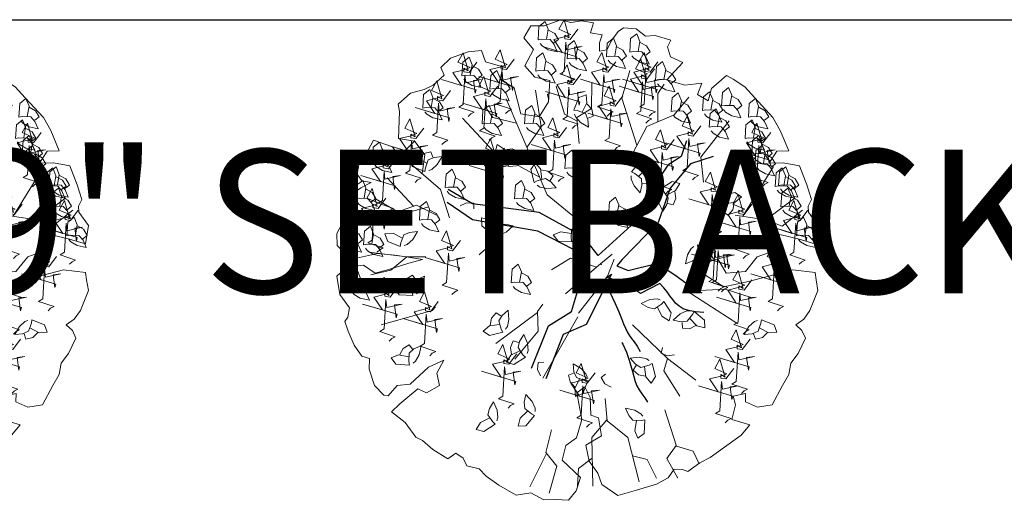
# Model space of a CAD drawing. Units: inches. Extents: x 2831 to 4250, y 1103 to 1797.
# Tile 8 of 15: x 3614 to 3676, y 1690 to 1721. Entities that reach past the tile are written whole.
import ezdxf

# ---------------------------------------------------------------- set-up
doc = ezdxf.new("R2010")
doc.units = ezdxf.units.IN
for name, color, linetype, lineweight in [('A-ANNO-DIMS', 2, 'Continuous', 18), ('A-ANNO-TEXT', 7, 'Continuous', 18), ('A-WALL-PATT', 252, 'Continuous', 13), ('ARBOL', 30, 'Continuous', 13), ('C-PROP', 7, 'Continuous', 25)]:
    doc.layers.add(name, color=color, linetype=linetype, lineweight=lineweight)
doc.layers.add('TALLO', color=36, linetype='Continuous')
doc.styles.get("Standard").update_dxf_attribs({"font": 'arial.ttf'})
doc.dimstyles.new('ISO-25', dxfattribs={"dimtxt": 9, "dimasz": 2.5, "dimexe": 1.25, "dimexo": 0.625, "dimtad": 1, "dimdec": 1, "dimlunit": 3, "dimtxsty": 'Standard', "dimcen": 2.5, "dimadec": 0, "dimazin": 0, "dimtfac": 1, "dimtdec": 1, "dimtmove": 0, "dimatfit": 3, "dimfxl": 1, "dimarcsym": 0})

# ---------------------------------------------------------------- blocks, each defined once
blk = doc.blocks.new('fresno')
at = {"layer": 'ARBOL'}
for p, q in [((2.96, 0.991), (3.575, 1.984)), ((-3.638, 1.194), (-4.164, 1.76)), ((-1.151, -0.932), (-1.99, -1.556)), ((-0.974, -3.757), (-1.31, -4.423))]:
    blk.add_line(p, q, dxfattribs=at)
blk.add_lwpolyline([(0.823, 4.745), (0.566, 4.764), (0.459, 4.687), (0.336, 4.518), (0.233, 4.322), (0.087, 4.298), (0.091, 4.464), (0.14, 4.621), (-0.09, 4.659), (-0.033, 4.863), (-0.264, 4.901), (-0.483, 4.866), (-0.686, 4.924), (-1.021, 4.801), (-1.288, 4.8), (-1.431, 4.563), (-1.234, 4.327), (-1.406, 4), (-1.205, 3.778), (-0.909, 3.705), (-0.931, 3.283), (-1.122, 2.983), (-1.491, 3.043), (-1.619, 3.562), (-1.9, 3.727), (-1.851, 3.982), (-2.197, 4.084), (-2.278, 4.31), (-2.543, 4.283), (-2.896, 4.152), (-3.091, 3.971), (-3.022, 3.817), (-3.244, 3.617), (-3.424, 3.528), (-3.697, 3.455), (-3.946, 3.236), (-3.922, 3.09), (-3.94, 2.548), (-3.617, 2.495), (-3.927, 2.19), (-4.062, 2.379), (-4.443, 2.512), (-4.546, 2.316), (-4.73, 2.062), (-4.767, 1.832), (-4.671, 1.698), (-4.486, 1.667), (-4.693, 1.559), (-4.854, 1.444), (-4.934, 1.102), (-5.037, 0.905), (-5.175, 0.644), (-5.166, 0.406), (-5.024, 0.264), (-4.781, 0.153), (-4.363, 0.249), (-4.014, 0.215), (-3.783, 0.177), (-3.46, 0.124), (-3.733, 0.051), (-4.132, -0.073), (-4.404, -0.146), (-4.639, 0.011), (-4.977, -0.028), (-5.172, -0.209), (-5.113, -0.574), (-4.921, -0.843), (-4.951, -1.027), (-5.012, -1.112), (-4.95, -1.311), (-4.83, -1.592), (-4.676, -1.807), (-4.518, -1.856), (-4.529, -2.068), (-4.417, -2.394), (-4.236, -2.59), (-4.143, -2.605), (-3.967, -2.397), (-3.703, -2.37), (-3.339, -2.027), (-3.032, -1.889), (-3.169, -2.15), (-3.115, -2.396), (-3.376, -2.542), (-3.552, -2.466), (-3.909, -2.762), (-4.077, -2.924), (-3.804, -3.135), (-3.592, -3.43), (-3.461, -3.499), (-3.253, -3.676), (-2.953, -3.867), (-2.792, -3.752), (-2.642, -3.848), (-2.572, -4.001), (-2.323, -4.066), (-2.18, -4.208), (-1.926, -4.392), (-1.58, -4.591), (-1.288, -4.545), (-1.027, -4.683), (-0.788, -4.675), (-0.531, -4.693), (-0.382, -4.505), (-0.29, -4.236), (-0.66, -3.891), (-0.588, -3.595), (-0.374, -3.441), (-0.267, -3.079), (-0.368, -2.541), (-0.208, -2.426), (-0.099, -2.633), (-0.087, -2.991), (0.071, -3.04), (0.129, -3.405), (-0.185, -3.59), (-0.119, -3.909), (0.055, -4.151), (0.136, -4.377), (0.456, -4.596), (0.828, -4.491), (1.227, -4.368), (1.461, -4.241), (1.583, -4.071), (1.748, -4.075), (1.86, -4.117), (2.101, -3.944), (2.308, -3.836), (2.925, -3.393), (3.101, -3.185), (2.74, -3.078), (2.812, -2.782), (2.769, -2.61), (3.015, -2.555), (3.012, -2.721), (3.254, -2.832), (3.546, -2.785), (3.752, -2.393), (3.882, -2.177), (3.92, -1.947), (4.069, -1.758), (4.214, -1.451), (4.144, -1.297), (4.021, -1.182), (4.182, -1.067), (4.304, -0.897), (4.464, -0.497), (4.429, -0.279), (4.406, -0.133), (3.964, -0.083), (3.074, -0.315), (2.582, -0.424), (2.217, -0.197), (2.136, 0.029), (2.462, 0.141), (2.628, -0.147), (3.012, -0.116), (3.249, 0.177), (3.602, 0.308), (3.701, 0.623), (4.089, 0.535), (4.404, 0.436), (4.464, 0.805), (4.272, 1.074), (4.267, 1.193), (4.336, 1.324), (4.243, 1.623), (4.092, 2.003), (3.769, 2.057), (3.485, 2.056), (3.642, 2.291), (3.88, 2.299), (3.71, 2.706), (3.563, 2.967), (3.201, 3.358), (3.001, 3.581), (2.766, 3.738), (2.635, 3.807), (2.332, 3.549), (2.268, 3.299), (2.052, 3.429), (2.136, 3.652), (1.798, 3.613), (1.437, 3.72), (1.755, 4.071), (1.513, 4.182), (1.451, 4.381), (1.519, 4.512), (1.204, 4.611), (1.012, 4.596)], close=True, dxfattribs=at)
for points in [[(-1.104, 4.45), (-1.063, 4.399), (-0.939, 4.325), (-0.757, 4.285), (-0.82, 4.431), (-0.903, 4.527), (-1.075, 4.533), (-1.143, 4.521), (-1.126, 4.792), (-1.002, 4.891), (-0.939, 4.738), (-0.975, 4.535)], [(-0.346, 4.735), (-0.501, 4.528), (-0.605, 4.545), (-0.605, 4.614), (-0.519, 4.563), (-0.622, 4.925), (-0.726, 4.735), (-0.484, 4.632), (-0.622, 4.58), (-0.829, 4.528), (-0.657, 4.27), (-1.053, 4.39), (-0.363, 4.183), (-0.381, 4.114), (-0.415, 4.373), (-0.26, 4.39), (-0.57, 4.321), (-0.588, 4.476), (-0.622, 3.89), (-0.708, 3.839), (-0.398, 3.735), (-0.467, 3.701), (-0.519, 3.649)], [(-0.935, 4.717), (-0.809, 4.65), (-0.736, 4.529), (-0.824, 4.459)], [(0.263, 4.114), (0.304, 4.063), (0.429, 3.989), (0.611, 3.948), (0.547, 4.095), (0.465, 4.191), (0.293, 4.197), (0.225, 4.185), (0.242, 4.456), (0.366, 4.555), (0.428, 4.402), (0.393, 4.199)], [(0.734, 4.203), (0.775, 4.152), (0.9, 4.078), (1.082, 4.038), (1.018, 4.185), (0.936, 4.281), (0.763, 4.287), (0.696, 4.274), (0.712, 4.546), (0.837, 4.645), (0.899, 4.491), (0.863, 4.289)], [(-0.521, 4.069), (-0.48, 4.018), (-0.356, 3.944), (-0.174, 3.904), (-0.237, 4.051), (-0.32, 4.146), (-0.492, 4.152), (-0.56, 4.14), (-0.543, 4.411), (-0.419, 4.511), (-0.356, 4.357), (-0.392, 4.154)], [(0.433, 4.381), (0.558, 4.314), (0.631, 4.193), (0.544, 4.122)], [(0.904, 4.471), (1.029, 4.404), (1.102, 4.282), (1.015, 4.212)], [(-2.368, 4.073), (-2.523, 3.866), (-2.627, 3.883), (-2.627, 3.952), (-2.541, 3.9), (-2.644, 4.262), (-2.748, 4.073), (-2.506, 3.969), (-2.644, 3.918), (-2.851, 3.866), (-2.679, 3.607), (-3.075, 3.728), (-2.385, 3.521), (-2.403, 3.452), (-2.437, 3.711), (-2.282, 3.728), (-2.592, 3.659), (-2.61, 3.814), (-2.644, 3.228), (-2.73, 3.176), (-2.42, 3.073), (-2.489, 3.038), (-2.541, 2.987)], [(-2.629, 3.733), (-2.588, 3.682), (-2.463, 3.608), (-2.281, 3.568), (-2.345, 3.715), (-2.427, 3.81), (-2.6, 3.816), (-2.667, 3.804), (-2.651, 4.075), (-2.526, 4.175), (-2.464, 4.021), (-2.5, 3.818)], [(-1.623, 4.132), (-1.778, 3.925), (-1.882, 3.942), (-1.882, 4.011), (-1.795, 3.959), (-1.899, 4.321), (-2.002, 4.132), (-1.761, 4.028), (-1.899, 3.977), (-2.106, 3.925), (-1.933, 3.666), (-2.33, 3.787), (-1.64, 3.58), (-1.657, 3.511), (-1.692, 3.77), (-1.537, 3.787), (-1.847, 3.718), (-1.864, 3.873), (-1.899, 3.287), (-1.985, 3.235), (-1.675, 3.132), (-1.744, 3.097), (-1.795, 3.046)], [(-1.149, 3.822), (-1.108, 3.771), (-0.983, 3.697), (-0.802, 3.657), (-0.865, 3.804), (-0.948, 3.9), (-1.12, 3.906), (-1.188, 3.893), (-1.171, 4.165), (-1.047, 4.264), (-0.984, 4.111), (-1.02, 3.908)], [(-0.352, 4.337), (-0.226, 4.269), (-0.153, 4.148), (-0.241, 4.078)], [(0.413, 4.08), (0.258, 3.873), (0.154, 3.89), (0.154, 3.959), (0.241, 3.908), (0.137, 4.27), (0.034, 4.08), (0.275, 3.977), (0.137, 3.925), (-0.07, 3.873), (0.103, 3.614), (-0.294, 3.735), (0.396, 3.528), (0.379, 3.459), (0.344, 3.718), (0.499, 3.735), (0.189, 3.666), (0.172, 3.821), (0.137, 3.235), (0.051, 3.183), (0.361, 3.08), (0.292, 3.046), (0.241, 2.994)], [(1.259, 4.08), (1.103, 3.873), (1, 3.89), (1, 3.959), (1.086, 3.908), (0.982, 4.27), (0.879, 4.08), (1.12, 3.977), (0.982, 3.925), (0.775, 3.873), (0.948, 3.614), (0.551, 3.735), (1.241, 3.528), (1.224, 3.459), (1.189, 3.718), (1.345, 3.735), (1.034, 3.666), (1.017, 3.821), (0.982, 3.235), (0.896, 3.183), (1.207, 3.08), (1.138, 3.046), (1.086, 2.994)], [(-2.459, 4), (-2.334, 3.933), (-2.261, 3.812), (-2.348, 3.742)], [(-0.287, 3.833), (-0.442, 3.626), (-0.546, 3.643), (-0.546, 3.712), (-0.46, 3.661), (-0.563, 4.023), (-0.667, 3.833), (-0.425, 3.73), (-0.563, 3.678), (-0.77, 3.626), (-0.598, 3.367), (-0.995, 3.488), (-0.304, 3.281), (-0.322, 3.212), (-0.356, 3.471), (-0.201, 3.488), (-0.511, 3.419), (-0.529, 3.574), (-0.563, 2.988), (-0.649, 2.936), (-0.339, 2.833), (-0.408, 2.799), (-0.46, 2.747)], [(-0.98, 4.09), (-0.854, 4.023), (-0.781, 3.901), (-0.869, 3.831)], [(1.189, 3.942), (1.034, 3.735), (0.931, 3.752), (0.931, 3.821), (1.017, 3.77), (0.913, 4.132), (0.81, 3.942), (1.051, 3.839), (0.913, 3.787), (0.706, 3.735), (0.879, 3.477), (0.482, 3.597), (1.172, 3.39), (1.155, 3.321), (1.12, 3.58), (1.276, 3.597), (0.965, 3.528), (0.948, 3.683), (0.913, 3.097), (0.827, 3.046), (1.138, 2.942), (1.069, 2.908), (1.017, 2.856)], [(1.25, 3.643), (1.291, 3.592), (1.416, 3.518), (1.597, 3.478), (1.534, 3.625), (1.451, 3.721), (1.279, 3.727), (1.211, 3.714), (1.228, 3.985), (1.352, 4.085), (1.415, 3.931), (1.379, 3.729)], [(-1.951, 3.597), (-2.106, 3.39), (-2.209, 3.408), (-2.209, 3.477), (-2.123, 3.425), (-2.227, 3.787), (-2.33, 3.597), (-2.089, 3.494), (-2.227, 3.442), (-2.434, 3.39), (-2.261, 3.132), (-2.658, 3.252), (-1.968, 3.046), (-1.985, 2.977), (-2.02, 3.235), (-1.864, 3.252), (-2.175, 3.183), (-2.192, 3.339), (-2.227, 2.752), (-2.313, 2.701), (-2.002, 2.597), (-2.071, 2.563), (-2.123, 2.511)], [(-2.068, 3.464), (-2.027, 3.413), (-1.903, 3.339), (-1.721, 3.299), (-1.784, 3.446), (-1.867, 3.542), (-2.039, 3.547), (-2.107, 3.535), (-2.09, 3.806), (-1.966, 3.906), (-1.903, 3.752), (-1.939, 3.55)], [(0.837, 2.414), (0.533, 3.352), (0.697, 3.906)], [(1.419, 3.911), (1.545, 3.844), (1.618, 3.722), (1.53, 3.652)], [(-2.898, 3.511), (-3.053, 3.304), (-3.157, 3.321), (-3.157, 3.39), (-3.071, 3.339), (-3.174, 3.701), (-3.278, 3.511), (-3.036, 3.408), (-3.174, 3.356), (-3.381, 3.304), (-3.209, 3.046), (-3.605, 3.166), (-2.915, 2.959), (-2.932, 2.89), (-2.967, 3.149), (-2.812, 3.166), (-3.122, 3.097), (-3.14, 3.253), (-3.174, 2.666), (-3.26, 2.615), (-2.95, 2.511), (-3.019, 2.477), (-3.071, 2.425)], [(-1.899, 3.732), (-1.773, 3.664), (-1.7, 3.543), (-1.788, 3.473)], [(-0.358, 2.895), (-0.615, 3.037), (-0.783, 3.596)], [(-0.063, 3.671), (-0.069, 3.151), (-0.364, 2.965), (-0.319, 2.449)], [(0.558, 3.402), (0.403, 3.195), (0.299, 3.212), (0.299, 3.281), (0.386, 3.23), (0.282, 3.592), (0.179, 3.402), (0.42, 3.299), (0.282, 3.247), (0.075, 3.195), (0.248, 2.936), (-0.149, 3.057), (0.541, 2.85), (0.524, 2.781), (0.489, 3.04), (0.644, 3.057), (0.334, 2.988), (0.317, 3.143), (0.282, 2.557), (0.196, 2.505), (0.506, 2.402), (0.437, 2.368), (0.386, 2.316)], [(1.259, 2.882), (1.254, 3.446), (1.381, 3.636)], [(2.573, 3.128), (2.613, 3.077), (2.738, 3.003), (2.92, 2.963), (2.857, 3.11), (2.774, 3.205), (2.602, 3.211), (2.534, 3.199), (2.551, 3.47), (2.675, 3.57), (2.738, 3.416), (2.702, 3.214)], [(-3.413, 3.083), (-3.373, 3.032), (-3.248, 2.958), (-3.066, 2.918), (-3.129, 3.065), (-3.212, 3.161), (-3.384, 3.167), (-3.452, 3.154), (-3.435, 3.425), (-3.311, 3.525), (-3.248, 3.371), (-3.284, 3.169)], [(-1.367, 2.367), (-1.081, 2.78), (-1.193, 3.514)], [(-0.923, 3.449), (-0.951, 3.425), (-0.93, 3.313)], [(-0.41, 3.035), (-0.387, 2.974), (-0.291, 2.865), (-0.131, 2.771), (-0.146, 2.93), (-0.195, 3.047), (-0.357, 3.106), (-0.425, 3.115), (-0.325, 3.368), (-0.176, 3.424), (-0.164, 3.258), (-0.261, 3.077)], [(0.746, 2.242), (1.034, 2.786), (1.584, 3.019), (1.879, 3.374)], [(1.564, 3.016), (1.605, 2.965), (1.729, 2.891), (1.911, 2.851), (1.848, 2.998), (1.765, 3.094), (1.593, 3.099), (1.525, 3.087), (1.542, 3.358), (1.666, 3.458), (1.729, 3.304), (1.693, 3.102)], [(2.191, 3.038), (2.232, 2.987), (2.357, 2.913), (2.539, 2.873), (2.475, 3.02), (2.393, 3.116), (2.221, 3.122), (2.153, 3.109), (2.17, 3.381), (2.294, 3.48), (2.356, 3.326), (2.321, 3.124)], [(2.742, 3.396), (2.868, 3.328), (2.941, 3.207), (2.853, 3.137)], [(-3.244, 3.351), (-3.118, 3.284), (-3.045, 3.162), (-3.133, 3.092)], [(-2.225, 2.77), (-2.184, 2.718), (-2.06, 2.645), (-1.878, 2.604), (-1.941, 2.751), (-2.024, 2.847), (-2.196, 2.853), (-2.264, 2.84), (-2.247, 3.112), (-2.123, 3.211), (-2.06, 3.058), (-2.096, 2.855)], [(-1.575, 2.854), (-2.052, 2.969), (-2.2, 3.178)], [(-0.448, 1), (-0.961, 1.419), (-1.784, 3.341)], [(-1.373, 2.77), (-1.332, 2.718), (-1.208, 2.645), (-1.026, 2.604), (-1.089, 2.751), (-1.172, 2.847), (-1.344, 2.853), (-1.412, 2.84), (-1.395, 3.112), (-1.271, 3.211), (-1.208, 3.058), (-1.244, 2.855)], [(-0.166, 3.238), (-0.068, 3.135), (-0.036, 2.997), (-0.141, 2.957)], [(1.733, 3.284), (1.859, 3.216), (1.932, 3.095), (1.844, 3.025)], [(2.361, 3.306), (2.486, 3.239), (2.559, 3.117), (2.472, 3.047)], [(3.111, 2.904), (3.152, 2.853), (3.276, 2.779), (3.458, 2.739), (3.395, 2.886), (3.312, 2.981), (3.14, 2.987), (3.072, 2.975), (3.089, 3.246), (3.213, 3.346), (3.276, 3.192), (3.24, 2.99)], [(3.28, 3.172), (3.406, 3.104), (3.479, 2.983), (3.391, 2.913)], [(-2.056, 3.037), (-1.93, 2.97), (-1.857, 2.849), (-1.945, 2.778)], [(-0.57, 2.77), (-0.726, 2.563), (-0.829, 2.58), (-0.829, 2.649), (-0.743, 2.597), (-0.846, 2.959), (-0.95, 2.77), (-0.708, 2.666), (-0.846, 2.615), (-1.053, 2.563), (-0.881, 2.304), (-1.278, 2.425), (-0.588, 2.218), (-0.605, 2.149), (-0.639, 2.408), (-0.484, 2.425), (-0.795, 2.356), (-0.812, 2.511), (-0.846, 1.925), (-0.933, 1.873), (-0.622, 1.77), (-0.691, 1.735), (-0.743, 1.684)], [(-1.204, 3.037), (-1.078, 2.97), (-1.005, 2.849), (-1.093, 2.778)], [(2.121, 2.804), (1.966, 2.597), (1.862, 2.615), (1.862, 2.683), (1.949, 2.632), (1.845, 2.994), (1.742, 2.804), (1.983, 2.701), (1.845, 2.649), (1.638, 2.597), (1.811, 2.339), (1.414, 2.459), (2.104, 2.252), (2.087, 2.184), (2.052, 2.442), (2.207, 2.459), (1.897, 2.39), (1.88, 2.546), (1.845, 1.959), (1.759, 1.908), (2.069, 1.804), (2, 1.77), (1.949, 1.718)], [(2.326, 2.702), (2.367, 2.651), (2.492, 2.577), (2.673, 2.537), (2.61, 2.684), (2.527, 2.78), (2.355, 2.786), (2.287, 2.773), (2.304, 3.045), (2.428, 3.144), (2.491, 2.99), (2.455, 2.788)], [(2.495, 2.97), (2.621, 2.903), (2.694, 2.781), (2.606, 2.711)], [(-3.434, 2.752), (-3.59, 2.546), (-3.693, 2.563), (-3.693, 2.632), (-3.607, 2.58), (-3.71, 2.942), (-3.814, 2.752), (-3.572, 2.649), (-3.71, 2.597), (-3.917, 2.546), (-3.745, 2.287), (-4.142, 2.408), (-3.452, 2.201), (-3.469, 2.132), (-3.503, 2.39), (-3.348, 2.408), (-3.659, 2.339), (-3.676, 2.494), (-3.71, 1.908), (-3.797, 1.856), (-3.486, 1.753), (-3.555, 1.718), (-3.607, 1.666)], [(-1.112, 1.773), (-2.014, 2.265), (-2.654, 2.957)], [(2.171, 1.674), (2.121, 2.172), (2.689, 2.898)], [(3.519, 2.666), (3.363, 2.459), (3.26, 2.477), (3.26, 2.546), (3.346, 2.494), (3.243, 2.856), (3.139, 2.666), (3.381, 2.563), (3.243, 2.511), (3.036, 2.459), (3.208, 2.201), (2.811, 2.321), (3.501, 2.115), (3.484, 2.046), (3.45, 2.304), (3.605, 2.321), (3.294, 2.252), (3.277, 2.408), (3.243, 1.821), (3.156, 1.77), (3.467, 1.666), (3.398, 1.632), (3.346, 1.58)], [(3.043, 2.478), (3.084, 2.427), (3.209, 2.353), (3.391, 2.313), (3.327, 2.46), (3.245, 2.556), (3.073, 2.562), (3.005, 2.549), (3.022, 2.82), (3.146, 2.92), (3.208, 2.766), (3.173, 2.564)], [(1.586, 2.528), (1.431, 2.321), (1.327, 2.339), (1.327, 2.408), (1.414, 2.356), (1.31, 2.718), (1.207, 2.528), (1.448, 2.425), (1.31, 2.373), (1.103, 2.321), (1.276, 2.063), (0.879, 2.184), (1.569, 1.977), (1.552, 1.908), (1.517, 2.166), (1.673, 2.184), (1.362, 2.115), (1.345, 2.27), (1.31, 1.684), (1.224, 1.632), (1.535, 1.528), (1.466, 1.494), (1.414, 1.442)], [(3.178, 2.165), (3.219, 2.113), (3.344, 2.04), (3.525, 1.999), (3.462, 2.146), (3.379, 2.242), (3.207, 2.248), (3.139, 2.236), (3.156, 2.507), (3.28, 2.606), (3.343, 2.453), (3.307, 2.25)], [(3.213, 2.746), (3.338, 2.679), (3.411, 2.557), (3.324, 2.487)], [(-4.422, 2.03), (-4.381, 1.979), (-4.257, 1.905), (-4.075, 1.865), (-4.138, 2.012), (-4.221, 2.108), (-4.393, 2.114), (-4.461, 2.101), (-4.444, 2.372), (-4.32, 2.472), (-4.257, 2.318), (-4.293, 2.116)], [(-3.468, 1.85), (-3.409, 2.222), (-3.628, 2.505)], [(-1.817, 2.351), (-1.972, 2.144), (-2.075, 2.162), (-2.075, 2.231), (-1.989, 2.179), (-2.093, 2.541), (-2.196, 2.351), (-1.955, 2.248), (-2.093, 2.196), (-2.3, 2.144), (-2.127, 1.886), (-2.524, 2.006), (-1.834, 1.8), (-1.851, 1.731), (-1.886, 1.989), (-1.73, 2.006), (-2.041, 1.937), (-2.058, 2.093), (-2.093, 1.506), (-2.179, 1.455), (-1.868, 1.351), (-1.937, 1.317), (-1.989, 1.265)], [(-1.786, 2.007), (-1.722, 1.99), (-1.578, 2.003), (-1.407, 2.078), (-1.545, 2.159), (-1.668, 2.188), (-1.811, 2.092), (-1.859, 2.042), (-2.004, 2.271), (-1.962, 2.425), (-1.821, 2.337), (-1.731, 2.152)], [(3.245, 1.963), (3.286, 1.912), (3.411, 1.838), (3.593, 1.798), (3.529, 1.945), (3.447, 2.041), (3.274, 2.046), (3.206, 2.034), (3.223, 2.305), (3.347, 2.405), (3.41, 2.251), (3.374, 2.049)], [(3.347, 2.432), (3.473, 2.365), (3.546, 2.244), (3.458, 2.173)], [(-3.986, 2.149), (-4.142, 1.942), (-4.245, 1.959), (-4.245, 2.028), (-4.159, 1.977), (-4.262, 2.339), (-4.366, 2.149), (-4.124, 2.046), (-4.262, 1.994), (-4.47, 1.942), (-4.297, 1.684), (-4.694, 1.804), (-4.004, 1.597), (-4.021, 1.528), (-4.055, 1.787), (-3.9, 1.804), (-4.211, 1.735), (-4.228, 1.89), (-4.262, 1.304), (-4.349, 1.253), (-4.038, 1.149), (-4.107, 1.115), (-4.159, 1.063)], [(-4.253, 2.298), (-4.127, 2.231), (-4.054, 2.109), (-4.142, 2.039)], [(-2.916, 0.958), (-3.096, 1.528), (-3.871, 2.197)], [(-3.331, 1.905), (-3.269, 1.928), (-3.161, 2.024), (-3.066, 2.184), (-3.226, 2.169), (-3.342, 2.121), (-3.401, 1.958), (-3.41, 1.89), (-3.663, 1.99), (-3.719, 2.139), (-3.554, 2.151), (-3.372, 2.054)], [(-3.533, 2.149), (-3.43, 2.247), (-3.292, 2.279), (-3.252, 2.174)], [(-1.806, 2.323), (-1.665, 2.343), (-1.534, 2.287), (-1.564, 2.179)], [(-0.566, 1.873), (-0.525, 1.822), (-0.4, 1.748), (-0.219, 1.708), (-0.282, 1.855), (-0.365, 1.951), (-0.537, 1.957), (-0.605, 1.944), (-0.588, 2.216), (-0.464, 2.315), (-0.401, 2.162), (-0.437, 1.959)], [(3.415, 2.231), (3.54, 2.163), (3.613, 2.042), (3.525, 1.972)], [(-1.164, 1.612), (-1.109, 1.576), (-0.967, 1.544), (-0.782, 1.562), (-0.888, 1.682), (-0.996, 1.748), (-1.162, 1.7), (-1.222, 1.667), (-1.29, 1.93), (-1.203, 2.063), (-1.096, 1.937), (-1.067, 1.733)], [(-0.397, 2.141), (-0.271, 2.074), (-0.198, 1.952), (-0.286, 1.882)], [(0.72, 1.798), (0.723, 1.733), (0.781, 1.6), (0.904, 1.46), (0.939, 1.616), (0.929, 1.742), (0.793, 1.848), (0.73, 1.878), (0.904, 2.088), (1.062, 2.095), (1.023, 1.934), (0.875, 1.791)], [(3.716, 1.537), (3.757, 1.486), (3.882, 1.412), (4.063, 1.372), (4, 1.519), (3.917, 1.615), (3.745, 1.621), (3.677, 1.608), (3.694, 1.88), (3.818, 1.979), (3.881, 1.825), (3.845, 1.623)], [(-2.965, 1.493), (-2.924, 1.441), (-2.799, 1.368), (-2.618, 1.327), (-2.681, 1.474), (-2.764, 1.57), (-2.936, 1.576), (-3.004, 1.564), (-2.987, 1.835), (-2.863, 1.934), (-2.8, 1.781), (-2.836, 1.578)], [(-1.085, 1.919), (-0.945, 1.893), (-0.838, 1.801), (-0.9, 1.707)], [(1.014, 1.915), (1.077, 1.787), (1.064, 1.646), (0.952, 1.64)], [(2.587, 1.684), (2.432, 1.477), (2.328, 1.494), (2.328, 1.563), (2.414, 1.511), (2.311, 1.873), (2.207, 1.684), (2.449, 1.58), (2.311, 1.528), (2.104, 1.477), (2.276, 1.218), (1.88, 1.339), (2.57, 1.132), (2.552, 1.063), (2.518, 1.321), (2.673, 1.339), (2.363, 1.27), (2.345, 1.425), (2.311, 0.839), (2.225, 0.787), (2.535, 0.684), (2.466, 0.649), (2.414, 0.597)], [(3.649, 1.515), (3.69, 1.464), (3.814, 1.39), (3.996, 1.35), (3.933, 1.497), (3.85, 1.592), (3.678, 1.598), (3.61, 1.586), (3.627, 1.857), (3.751, 1.957), (3.814, 1.803), (3.778, 1.601)], [(3.818, 1.783), (3.944, 1.715), (4.017, 1.594), (3.929, 1.524)], [(3.885, 1.805), (4.011, 1.738), (4.084, 1.616), (3.996, 1.546)], [(-4.759, 1.269), (-4.718, 1.217), (-4.593, 1.144), (-4.411, 1.103), (-4.475, 1.25), (-4.557, 1.346), (-4.729, 1.352), (-4.797, 1.339), (-4.78, 1.611), (-4.656, 1.71), (-4.594, 1.557), (-4.629, 1.354)], [(-2.796, 1.76), (-2.67, 1.693), (-2.597, 1.572), (-2.685, 1.501)], [(-1.575, 1.269), (-1.534, 1.217), (-1.409, 1.144), (-1.228, 1.103), (-1.291, 1.25), (-1.373, 1.346), (-1.546, 1.352), (-1.614, 1.339), (-1.597, 1.611), (-1.473, 1.71), (-1.41, 1.557), (-1.446, 1.354)], [(1.283, 1.469), (1.266, 1.405), (1.279, 1.261), (1.354, 1.09), (1.435, 1.228), (1.464, 1.351), (1.368, 1.494), (1.318, 1.542), (1.547, 1.687), (1.7, 1.645), (1.613, 1.504), (1.428, 1.414)], [(-4.193, 1.356), (-4.349, 1.149), (-4.452, 1.166), (-4.452, 1.235), (-4.366, 1.184), (-4.469, 1.546), (-4.573, 1.356), (-4.331, 1.253), (-4.469, 1.201), (-4.677, 1.149), (-4.504, 0.89), (-4.901, 1.011), (-4.211, 0.804), (-4.228, 0.735), (-4.262, 0.994), (-4.107, 1.011), (-4.418, 0.942), (-4.435, 1.097), (-4.469, 0.511), (-4.556, 0.459), (-4.245, 0.356), (-4.314, 0.322), (-4.366, 0.27)], [(-4.589, 1.536), (-4.464, 1.469), (-4.391, 1.348), (-4.478, 1.277)], [(-1.406, 1.536), (-1.28, 1.469), (-1.207, 1.348), (-1.295, 1.277)], [(1.599, 1.489), (1.618, 1.348), (1.563, 1.217), (1.455, 1.247)], [(2.479, 1.34), (2.443, 1.285), (2.411, 1.143), (2.429, 0.958), (2.549, 1.064), (2.615, 1.172), (2.567, 1.338), (2.534, 1.398), (2.797, 1.466), (2.93, 1.379), (2.804, 1.272), (2.6, 1.243)], [(3.139, 1.235), (2.984, 1.028), (2.88, 1.046), (2.88, 1.115), (2.967, 1.063), (2.863, 1.425), (2.759, 1.235), (3.001, 1.132), (2.863, 1.08), (2.656, 1.028), (2.828, 0.77), (2.432, 0.891), (3.122, 0.684), (3.105, 0.615), (3.07, 0.873), (3.225, 0.891), (2.915, 0.822), (2.897, 0.977), (2.863, 0.391), (2.777, 0.339), (3.087, 0.235), (3.018, 0.201), (2.967, 0.149)], [(3.761, 1.112), (3.802, 1.061), (3.926, 0.987), (4.108, 0.947), (4.045, 1.093), (3.962, 1.189), (3.79, 1.195), (3.722, 1.183), (3.739, 1.454), (3.863, 1.553), (3.926, 1.4), (3.89, 1.197)], [(-3.192, 1.017), (-3.578, 1.215), (-3.949, 1.081), (-4.398, 1.339)], [(-3.481, 0.843), (-3.44, 0.792), (-3.315, 0.718), (-3.133, 0.678), (-3.197, 0.825), (-3.279, 0.92), (-3.451, 0.926), (-3.519, 0.914), (-3.502, 1.185), (-3.378, 1.285), (-3.316, 1.131), (-3.351, 0.928)], [(-2.703, 1.201), (-2.575, 1.263), (-2.433, 1.251), (-2.428, 1.139)], [(0.308, 0.933), (0.349, 0.881), (0.474, 0.807), (0.656, 0.767), (0.592, 0.914), (0.51, 1.01), (0.337, 1.016), (0.27, 1.003), (0.286, 1.275), (0.411, 1.374), (0.473, 1.221), (0.437, 1.018)], [(0.478, 1.2), (0.603, 1.133), (0.676, 1.011), (0.589, 0.941)], [(2.786, 1.261), (2.76, 1.121), (2.668, 1.014), (2.574, 1.076)], [(4.01, 1.36), (3.422, 0.918)], [(4.26, 1.115), (4.105, 0.908), (4.002, 0.925), (4.002, 0.994), (4.088, 0.942), (3.984, 1.304), (3.881, 1.115), (4.122, 1.011), (3.984, 0.959), (3.777, 0.908), (3.95, 0.649), (3.553, 0.77), (4.243, 0.563), (4.226, 0.494), (4.191, 0.753), (4.347, 0.77), (4.036, 0.701), (4.019, 0.856), (3.984, 0.27), (3.898, 0.218), (4.209, 0.115), (4.14, 0.08), (4.088, 0.029)], [(3.93, 1.379), (4.056, 1.312), (4.129, 1.191), (4.041, 1.121)], [(-3.354, 1.176), (-4.529, 0.864)], [(-3.311, 1.111), (-3.186, 1.043), (-3.113, 0.922), (-3.2, 0.852)], [(2.808, 1.015), (3.422, 0.918), (3.422, 0.918), (3.748, 0.794), (4.154, 1.111)], [(-5.028, 0.44), (-4.987, 0.388), (-4.862, 0.315), (-4.68, 0.274), (-4.744, 0.421), (-4.826, 0.517), (-4.998, 0.523), (-5.066, 0.511), (-5.049, 0.782), (-4.925, 0.881), (-4.863, 0.728), (-4.898, 0.525)], [(-4.602, 0.35), (-4.561, 0.299), (-4.436, 0.225), (-4.254, 0.185), (-4.318, 0.332), (-4.4, 0.428), (-4.572, 0.433), (-4.64, 0.421), (-4.623, 0.692), (-4.499, 0.792), (-4.437, 0.638), (-4.472, 0.436)], [(-1.981, 0.615), (-1.915, 0.618), (-1.782, 0.676), (-1.643, 0.799), (-1.799, 0.834), (-1.925, 0.824), (-2.031, 0.688), (-2.061, 0.626), (-2.27, 0.799), (-2.278, 0.958), (-2.117, 0.918), (-1.974, 0.77)], [(-0.397, 0.517), (-0.346, 0.557), (-0.272, 0.682), (-0.232, 0.864), (-0.379, 0.801), (-0.474, 0.718), (-0.48, 0.546), (-0.468, 0.478), (-0.739, 0.495), (-0.838, 0.619), (-0.685, 0.682), (-0.482, 0.646)], [(4.075, 0.529), (4.116, 0.478), (4.24, 0.404), (4.422, 0.364), (4.359, 0.511), (4.276, 0.607), (4.104, 0.613), (4.036, 0.6), (4.053, 0.871), (4.177, 0.971), (4.24, 0.817), (4.204, 0.615)], [(4.244, 0.797), (4.37, 0.73), (4.443, 0.608), (4.355, 0.538)], [(-4.858, 0.707), (-4.733, 0.64), (-4.66, 0.519), (-4.747, 0.448)], [(-4.432, 0.618), (-4.307, 0.55), (-4.234, 0.429), (-4.321, 0.359)], [(-3.824, 0.404), (-3.763, 0.427), (-3.654, 0.523), (-3.559, 0.683), (-3.719, 0.668), (-3.835, 0.62), (-3.894, 0.457), (-3.903, 0.389), (-4.156, 0.489), (-4.212, 0.638), (-4.047, 0.65), (-3.865, 0.553)], [(-2.698, 0.509), (-2.854, 0.302), (-2.957, 0.319), (-2.957, 0.388), (-2.871, 0.336), (-2.974, 0.698), (-3.078, 0.509), (-2.836, 0.405), (-2.974, 0.353), (-3.182, 0.302), (-3.009, 0.043), (-3.406, 0.164), (-2.716, -0.043), (-2.733, -0.112), (-2.767, 0.147), (-2.612, 0.164), (-2.923, 0.095), (-2.94, 0.25), (-2.974, -0.336), (-3.061, -0.388), (-2.75, -0.491), (-2.819, -0.526), (-2.871, -0.577)], [(2.639, 0.58), (2.483, 0.373), (2.38, 0.391), (2.38, 0.46), (2.466, 0.408), (2.363, 0.77), (2.259, 0.58), (2.501, 0.477), (2.363, 0.425), (2.156, 0.373), (2.328, 0.115), (1.931, 0.235), (2.621, 0.029), (2.604, -0.04), (2.57, 0.218), (2.725, 0.235), (2.414, 0.166), (2.397, 0.322), (2.363, -0.265), (2.276, -0.316), (2.587, -0.42), (2.518, -0.454), (2.466, -0.506)], [(2.708, 0.563), (2.552, 0.356), (2.449, 0.373), (2.449, 0.442), (2.535, 0.391), (2.432, 0.753), (2.328, 0.563), (2.57, 0.46), (2.432, 0.408), (2.225, 0.356), (2.397, 0.097), (2, 0.218), (2.69, 0.011), (2.673, -0.058), (2.639, 0.201), (2.794, 0.218), (2.483, 0.149), (2.466, 0.304), (2.432, -0.282), (2.345, -0.334), (2.656, -0.437), (2.587, -0.471), (2.535, -0.523)], [(1.978, 0.384), (1.927, 0.343), (1.853, 0.218), (1.813, 0.036), (1.96, 0.1), (2.056, 0.182), (2.061, 0.355), (2.049, 0.422), (2.32, 0.406), (2.42, 0.281), (2.266, 0.219), (2.064, 0.254)], [(-3.394, 0.18), (-3.77, 0.182), (-4.532, 0.27)], [(-2.322, 0.222), (-2.219, 0.321), (-2.081, 0.353), (-2.042, 0.248)], [(-0.596, -0.564), (0.03, -0.026), (0.339, 0.235)], [(2.246, 0.214), (2.178, 0.089), (2.057, 0.016), (1.987, 0.103)], [(3.829, 0.184), (3.674, -0.023), (3.57, -0.006), (3.57, 0.063), (3.657, 0.011), (3.553, 0.373), (3.45, 0.184), (3.691, 0.08), (3.553, 0.029), (3.346, -0.023), (3.519, -0.282), (3.122, -0.161), (3.812, -0.368), (3.795, -0.437), (3.76, -0.178), (3.915, -0.161), (3.605, -0.23), (3.588, -0.075), (3.553, -0.661), (3.467, -0.713), (3.777, -0.816), (3.708, -0.851), (3.657, -0.902)], [(-3.77, 0.182), (-4.09, -0.088), (-4.494, -0.18)], [(-1.642, -0.412), (-1.601, -0.463), (-1.477, -0.537), (-1.295, -0.577), (-1.358, -0.43), (-1.441, -0.334), (-1.613, -0.328), (-1.681, -0.341), (-1.664, -0.069), (-1.54, 0.03), (-1.477, -0.124), (-1.513, -0.326)], [(0.03, -0.026), (-0.491, 0.154), (-0.871, -0.08)], [(0.38, 0.131), (0.248, -0.21), (-0.33, -0.951)], [(-4.871, -0.524), (-4.83, -0.575), (-4.705, -0.649), (-4.523, -0.689), (-4.587, -0.542), (-4.669, -0.446), (-4.841, -0.44), (-4.909, -0.453), (-4.893, -0.181), (-4.768, -0.082), (-4.706, -0.236), (-4.741, -0.438)], [(-3.848, -0.389), (-3.781, -0.264), (-3.659, -0.191), (-3.589, -0.278)], [(-1.473, -0.144), (-1.347, -0.211), (-1.274, -0.333), (-1.362, -0.403)], [(3.139, -0.282), (2.984, -0.489), (2.88, -0.471), (2.88, -0.402), (2.967, -0.454), (2.863, -0.092), (2.759, -0.282), (3.001, -0.385), (2.863, -0.437), (2.656, -0.489), (2.828, -0.747), (2.432, -0.627), (3.122, -0.834), (3.105, -0.902), (3.07, -0.644), (3.225, -0.627), (2.915, -0.696), (2.897, -0.54), (2.863, -1.127), (2.777, -1.178), (3.087, -1.282), (3.018, -1.316), (2.967, -1.368)], [(-4.701, -0.256), (-4.576, -0.323), (-4.503, -0.445), (-4.59, -0.515)], [(-3.952, -0.42), (-4.107, -0.627), (-4.211, -0.609), (-4.211, -0.54), (-4.124, -0.592), (-4.228, -0.23), (-4.331, -0.42), (-4.09, -0.523), (-4.228, -0.575), (-4.435, -0.627), (-4.262, -0.885), (-4.659, -0.765), (-3.969, -0.971), (-3.986, -1.04), (-4.021, -0.782), (-3.866, -0.765), (-4.176, -0.834), (-4.193, -0.678), (-4.228, -1.265), (-4.314, -1.316), (-4.004, -1.42), (-4.073, -1.454), (-4.124, -1.506)], [(-3.58, -0.559), (-3.529, -0.518), (-3.455, -0.393), (-3.415, -0.211), (-3.562, -0.275), (-3.658, -0.357), (-3.664, -0.53), (-3.651, -0.597), (-3.923, -0.581), (-4.022, -0.456), (-3.868, -0.394), (-3.666, -0.43)], [(-3.141, -0.713), (-3.296, -0.92), (-3.4, -0.902), (-3.4, -0.834), (-3.314, -0.885), (-3.417, -0.523), (-3.521, -0.713), (-3.279, -0.816), (-3.417, -0.868), (-3.624, -0.92), (-3.452, -1.178), (-3.848, -1.058), (-3.158, -1.265), (-3.175, -1.333), (-3.21, -1.075), (-3.055, -1.058), (-3.365, -1.127), (-3.383, -0.971), (-3.417, -1.558), (-3.503, -1.609), (-3.193, -1.713), (-3.262, -1.747), (-3.314, -1.799)], [(1.822, -0.495), (2.859, -1.165)], [(1.846, -0.51), (2.605, -0.469), (3.129, -0.637)], [(-1.047, -0.767), (-1.151, -0.913), (-1.144, -1.307), (-1.61, -1.871)], [(1.304, -0.681), (1.241, -0.664), (1.097, -0.678), (0.926, -0.752), (1.064, -0.833), (1.187, -0.862), (1.33, -0.766), (1.377, -0.716), (1.523, -0.945), (1.481, -1.099), (1.34, -1.011), (1.25, -0.826)], [(-3.195, -0.824), (-3.267, -0.898), (-4.285, -1.185)], [(-1.794, -1.268), (-1.758, -1.214), (-1.726, -1.072), (-1.744, -0.887), (-1.865, -0.993), (-1.93, -1.101), (-1.883, -1.266), (-1.85, -1.327), (-2.113, -1.395), (-2.246, -1.307), (-2.119, -1.2), (-1.916, -1.172)], [(-2.101, -1.19), (-2.076, -1.05), (-1.983, -0.943), (-1.889, -1.004)], [(1.903, -0.903), (1.837, -0.905), (1.704, -0.963), (1.565, -1.086), (1.721, -1.122), (1.847, -1.111), (1.953, -0.975), (1.983, -0.913), (2.192, -1.086), (2.2, -1.245), (2.039, -1.205), (1.896, -1.057)], [(-0.346, -1.024), (-1.05, -2.251)], [(2.02, -1.197), (1.891, -1.259), (1.75, -1.247), (1.745, -1.134)], [(3.253, -1.094), (3.192, -1.117), (3.083, -1.213), (2.988, -1.374), (3.148, -1.359), (3.264, -1.31), (3.323, -1.148), (3.332, -1.079), (3.585, -1.179), (3.641, -1.328), (3.476, -1.34), (3.294, -1.244)], [(-1.361, -1.756), (-1.343, -1.693), (-1.357, -1.548), (-1.431, -1.377), (-1.513, -1.515), (-1.542, -1.638), (-1.445, -1.781), (-1.395, -1.829), (-1.625, -1.974), (-1.778, -1.932), (-1.691, -1.791), (-1.506, -1.701)], [(0.748, -1.185), (1.452, -1.855), (2.021, -2.292)], [(3.105, -1.471), (2.949, -1.678), (2.846, -1.661), (2.846, -1.592), (2.932, -1.644), (2.829, -1.282), (2.725, -1.471), (2.967, -1.575), (2.829, -1.627), (2.621, -1.678), (2.794, -1.937), (2.397, -1.816), (3.087, -2.023), (3.07, -2.092), (3.036, -1.833), (3.191, -1.816), (2.88, -1.885), (2.863, -1.73), (2.829, -2.316), (2.742, -2.368), (3.053, -2.471), (2.984, -2.506), (2.932, -2.558)], [(3.455, -1.338), (3.352, -1.437), (3.214, -1.469), (3.175, -1.364)], [(-1.571, -1.764), (-1.726, -1.971), (-1.83, -1.954), (-1.83, -1.885), (-1.744, -1.937), (-1.847, -1.575), (-1.951, -1.764), (-1.709, -1.868), (-1.847, -1.92), (-2.054, -1.971), (-1.882, -2.23), (-2.278, -2.109), (-1.588, -2.316), (-1.605, -2.385), (-1.64, -2.127), (-1.485, -2.109), (-1.795, -2.178), (-1.813, -2.023), (-1.847, -2.609), (-1.933, -2.661), (-1.623, -2.764), (-1.692, -2.799), (-1.744, -2.851)], [(-1.677, -1.776), (-1.696, -1.635), (-1.641, -1.504), (-1.533, -1.534)], [(-3.648, -1.948), (-3.596, -1.907), (-3.523, -1.782), (-3.482, -1.6), (-3.629, -1.664), (-3.725, -1.746), (-3.731, -1.919), (-3.719, -1.986), (-3.99, -1.97), (-4.089, -1.845), (-3.936, -1.783), (-3.733, -1.819)], [(-3.915, -1.778), (-3.848, -1.653), (-3.727, -1.58), (-3.656, -1.667)], [(1.593, -1.781), (1.452, -1.801), (1.322, -1.746), (1.352, -1.637)], [(-1.092, -2.202), (-1.154, -2.074), (-1.142, -1.933), (-1.03, -1.928)], [(-0.001, -2.144), (-0.156, -2.351), (-0.26, -2.333), (-0.26, -2.264), (-0.174, -2.316), (-0.277, -1.954), (-0.381, -2.144), (-0.139, -2.247), (-0.277, -2.299), (-0.484, -2.351), (-0.312, -2.609), (-0.708, -2.489), (-0.018, -2.695), (-0.035, -2.764), (-0.07, -2.506), (0.085, -2.489), (-0.225, -2.558), (-0.243, -2.402), (-0.277, -2.989), (-0.363, -3.04), (-0.053, -3.144), (-0.122, -3.178), (-0.174, -3.23)], [(-0.161, -2.225), (-0.184, -2.163), (-0.28, -2.055), (-0.44, -1.96), (-0.425, -2.12), (-0.376, -2.236), (-0.214, -2.295), (-0.146, -2.304), (-0.246, -2.557), (-0.395, -2.613), (-0.407, -2.448), (-0.31, -2.266)], [(1.086, -1.899), (1.031, -1.863), (0.89, -1.831), (0.704, -1.849), (0.81, -1.969), (0.918, -2.035), (1.084, -1.987), (1.145, -1.954), (1.212, -2.218), (1.125, -2.35), (1.018, -2.224), (0.989, -2.02)], [(1.452, -1.855), (1.379, -2.105), (1.698, -2.609)], [(2.777, -2.058), (2.621, -2.264), (2.518, -2.247), (2.518, -2.178), (2.604, -2.23), (2.501, -1.868), (2.397, -2.058), (2.639, -2.161), (2.501, -2.213), (2.294, -2.264), (2.466, -2.523), (2.069, -2.402), (2.759, -2.609), (2.742, -2.678), (2.708, -2.42), (2.863, -2.402), (2.552, -2.471), (2.535, -2.316), (2.501, -2.902), (2.414, -2.954), (2.725, -3.057), (2.656, -3.092), (2.604, -3.144)], [(-0.405, -2.427), (-0.503, -2.324), (-0.535, -2.186), (-0.43, -2.146)], [(0.319, -2.428), (0.193, -2.361), (0.12, -2.239), (0.208, -2.169)], [(1.007, -2.206), (0.867, -2.181), (0.76, -2.088), (0.822, -1.994)], [(-1.966, -3.1), (-1.949, -3.037), (-1.962, -2.892), (-2.037, -2.722), (-2.118, -2.859), (-2.147, -2.982), (-2.051, -3.125), (-2.001, -3.173), (-2.23, -3.319), (-2.383, -3.277), (-2.296, -3.136), (-2.111, -3.046)], [(-1.201, -2.914), (-1.204, -2.849), (-1.262, -2.716), (-1.385, -2.576), (-1.42, -2.732), (-1.41, -2.858), (-1.274, -2.964), (-1.212, -2.994), (-1.385, -3.204), (-1.544, -3.211), (-1.504, -3.05), (-1.356, -2.907)], [(0.201, -2.655), (0.24, -3.105), (0.657, -3.436), (0.886, -4.322)], [(0.959, -3.012), (0.918, -2.961), (0.793, -2.887), (0.612, -2.847), (0.675, -2.994), (0.758, -3.089), (0.93, -3.095), (0.998, -3.083), (0.981, -3.354), (0.857, -3.453), (0.794, -3.3), (0.83, -3.097)], [(1.399, -2.886), (1.63, -3.612), (1.964, -3.708), (2.084, -3.964)], [(0.238, -3.084), (-0.067, -3.438), (-0.048, -4.412)], [(-0.923, -4.549), (-0.768, -4.012), (-0.99, -3.737), (-0.872, -3.28)], [(1.625, -3.596), (1.438, -3.858), (1.657, -4.248)], [(-0.059, -3.851), (-0.336, -4.054), (-0.355, -4.41)], [(0.752, -3.801), (1.042, -3.878), (1.233, -4.25)]]:
    blk.add_lwpolyline(points, dxfattribs=at)
for p in [(-0.308, 0.101), (0.124, 0.027)]:
    blk.add_point(p, dxfattribs=at)
at = {"layer": 'TALLO'}
for points in [[(1.829, 2.5), (1.722, 2.184), (1.454, 2.012), (1.213, 1.639), (0.944, 1.008), (0.06, 0.204), (-0.234, 0.577), (-1.119, 1.065), (-2.458, 1.237), (-2.941, 1.524)], [(2.364, 2.184), (1.909, 2.041), (1.507, 1.552), (1.266, 0.864), (0.542, 0.125), (0.433, 0.001), (0.662, -0.096), (1.228, 0.045), (1.455, -0.09), (1.644, -0.216), (1.8, -0.33), (1.931, -0.425), (2.042, -0.496), (2.141, -0.539)], [(-1.272, -2.047), (-0.931, -1.203), (-0.475, -0.916), (-0.234, -0.112), (-0.422, 0.318), (-1.146, 0.691), (-2.458, 0.921), (-2.967, 1.266)], [(2.177, -0.932), (2.008, -0.924), (1.873, -0.898), (1.766, -0.859), (1.682, -0.807), (1.613, -0.745), (1.554, -0.676), (1.499, -0.6), (1.442, -0.521), (1.376, -0.44), (1.298, -0.357), (0.908, -0.555), (0.791, -0.474), (0.647, -0.394), (0.474, -0.317), (0.265, -0.244), (0.226, -0.233), (0.328, -0.17), (-0.181, -1.175), (-0.637, -1.375), (-0.985, -2.265)], [(0.219, -0.386), (0.3, -0.544), (0.399, -0.753), (0.473, -0.922), (0.529, -1.057), (0.571, -1.164), (0.607, -1.251), (0.641, -1.324), (0.68, -1.389), (0.729, -1.454), (0.784, -1.525), (0.844, -1.61), (0.903, -1.717)], [(0.538, -1.536), (0.555, -1.568), (0.626, -1.728), (0.678, -1.871), (0.716, -2), (0.747, -2.115), (0.773, -2.219), (0.802, -2.314), (0.837, -2.401), (0.883, -2.483), (0.936, -2.562), (0.994, -2.642), (1.052, -2.727)]]:
    blk.add_lwpolyline(points, dxfattribs=at)
blk = doc.blocks.new('*D77')
at = {"layer": 'A-ANNO-DIMS', "color": 0, "lineweight": -2, "transparency": 16777216}
for p, q in [((3512.227, 1679.888), (3512.227, 1668.463)), ((3584.227, 1679.888), (3584.227, 1668.463)), ((3514.727, 1669.713), (3581.727, 1669.713)), ((3584.227, 1669.713), (3701.864, 1669.713))]:
    blk.add_line(p, q, dxfattribs=at)
at = {"layer": 'A-ANNO-DIMS', "color": 0, "transparency": 16777216}
for points in [[(3514.727, 1670.13), (3514.727, 1669.297), (3512.227, 1669.713)], [(3581.727, 1670.13), (3581.727, 1669.297), (3584.227, 1669.713)]]:
    blk.add_solid(points, dxfattribs=at)
at = {"layer": 'Defpoints', "color": 0, "transparency": 16777216}
for p in [(3512.227, 1680.513), (3584.227, 1680.513), (3584.227, 1669.713)]:
    blk.add_point(p, dxfattribs=at)
at = {"layer": 'A-ANNO-DIMS', "color": 0, "transparency": 16777216, "insert": (3644.295, 1674.995), "char_height": 9, "attachment_point": 5}
blk.add_mtext('WINDOW 6\'-0" TYP.', dxfattribs=at)

msp = doc.modelspace()

# ---------------------------------------------------------------- hatches: boundary and pattern name
at = {"layer": 'A-WALL-PATT'}
h = msp.add_hatch(color=256, dxfattribs=at)
h.dxf.hatch_style = 1
h.paths.add_polyline_path([(3479.227, 1418.513), (3488.227, 1418.513), (3488.227, 1426.809), (3488.227, 1460.513), (3588.227, 1460.513), (3588.227, 1466.513), (3488.227, 1466.513), (3488.227, 1470.513), (3479.227, 1470.513)])
h.paths.add_polyline_path([(3488.227, 1506.513), (3488.227, 1512.513), (3479.227, 1512.513), (3479.227, 1506.513)])
h.paths.add_polyline_path([(3488.227, 1370.513), (3479.227, 1370.513), (3479.227, 1319.513), (3521.227, 1319.513), (3521.227, 1328.513), (3488.227, 1328.513)])
h.paths.add_polyline_path([(3794.227, 1319.513), (3794.227, 1247.513), (3614.227, 1247.513), (3614.227, 1242.513), (3803.227, 1242.513), (3803.227, 1328.513), (3767.227, 1328.513), (3767.227, 1394.513), (3758.227, 1394.513), (3758.227, 1328.513), (3635.227, 1328.513), (3635.227, 1460.513), (3637.227, 1460.513), (3637.227, 1466.513), (3624.227, 1466.513), (3624.227, 1460.513), (3626.227, 1460.513), (3626.227, 1328.513), (3593.227, 1328.513), (3593.227, 1319.513)])
h.paths.add_polyline_path([(3758.227, 1460.513), (3758.227, 1442.513), (3767.227, 1442.513), (3767.227, 1460.513), (3783.227, 1460.513), (3783.227, 1492.513), (3774.227, 1492.513), (3774.227, 1466.513), (3761.32, 1466.513), (3726.227, 1466.513), (3726.227, 1468.513), (3720.227, 1468.513), (3720.227, 1466.513), (3673.227, 1466.513), (3673.227, 1460.513)])
h.paths.add_polyline_path([(3597.627, 1698.243), (3687.215, 1698.243), (3687.215, 1717.459), (3597.627, 1717.459)], flags=9)
h.paths.add_polyline_path([(3776.749, 1438.286), (3776.749, 1360.767), (3795.966, 1360.767), (3795.966, 1438.286)], flags=25)
h.paths.add_polyline_path([(3453.373, 1482.946), (3453.373, 1401.852), (3472.59, 1401.852), (3472.59, 1482.946)], flags=9)
h.paths.add_polyline_path([(3506.208, 1267.098), (3560.706, 1267.098), (3560.706, 1293.711), (3506.208, 1293.711)], flags=9)
h.paths.add_polyline_path([(3760.502, 1579.698), (3798.745, 1579.698), (3798.745, 1602.509), (3760.502, 1602.509)], flags=9)
h.paths.add_polyline_path([(3617.004, 1637.953), (3659.123, 1637.953), (3659.123, 1660.764), (3617.004, 1660.764)], flags=9)
h.paths.add_polyline_path([(3679.387, 1612.632), (3728.455, 1612.632), (3728.455, 1639.245), (3679.387, 1639.245)], flags=9)
h.paths.add_polyline_path([(3731.075, 1499.721), (3773.194, 1499.721), (3773.194, 1522.532), (3731.075, 1522.532)], flags=9)
h.paths.add_polyline_path([(3652.819, 1496.485), (3701.947, 1496.485), (3701.947, 1523.098), (3652.819, 1523.098)], flags=9)
h.paths.add_polyline_path([(3550.367, 1510.971), (3604.502, 1510.971), (3604.502, 1537.584), (3550.367, 1537.584)], flags=9)
h.paths.add_polyline_path([(3514.446, 1612.632), (3570.67, 1612.632), (3570.67, 1639.245), (3514.446, 1639.245)], flags=9)

# ---------------------------------------------------------------- linework, layer by layer
at = {"layer": 'C-PROP'}
msp.add_lwpolyline([(3445.227, 1244.513), (3445.227, 1720.513), (3801.227, 1720.513)], dxfattribs=at)

# ---------------------------------------------------------------- block references
at = {"layer": 'ARBOL', "xscale": 3.132679885015571, "yscale": 3.132679885015571, "zscale": 3.132679885015571}
for p in [(3604.551, 1705.093), (3650.341, 1705.093)]:
    msp.add_blockref('fresno', p, dxfattribs=at)

# ---------------------------------------------------------------- texts
at = {"layer": 'A-ANNO-TEXT', "insert": (3600.163, 1712.367), "char_height": 9, "attachment_point": 1}
msp.add_mtext_dynamic_manual_height_columns('{\\fTimes New Roman|b0|i0|c0|p18;2\'9" SETBACK}', width=97.56899, gutter_width=12.5, heights=[0], dxfattribs=at)

# ---------------------------------------------------------------- dimensions: what is measured, and where the dimension line sits
at = {"layer": 'A-ANNO-DIMS'}
dim = msp.add_linear_dim(base=(3584.227, 1669.713), p1=(3512.227, 1680.513), p2=(3584.227, 1680.513), text='WINDOW <> TYP.', dimstyle='ISO-25', override={"dimdec": 1, "dimlfac": 1, "dimrnd": 0, "dimzin": 1, "dimdsep": 46, "dimlunit": 4, "dimfrac": 2}, dxfattribs=at)
dim.commit()
dim.dimension.update_dxf_attribs({"geometry": '*D77', "text_midpoint": (3644.295, 1674.995)})

doc.saveas('drawing.dxf')
